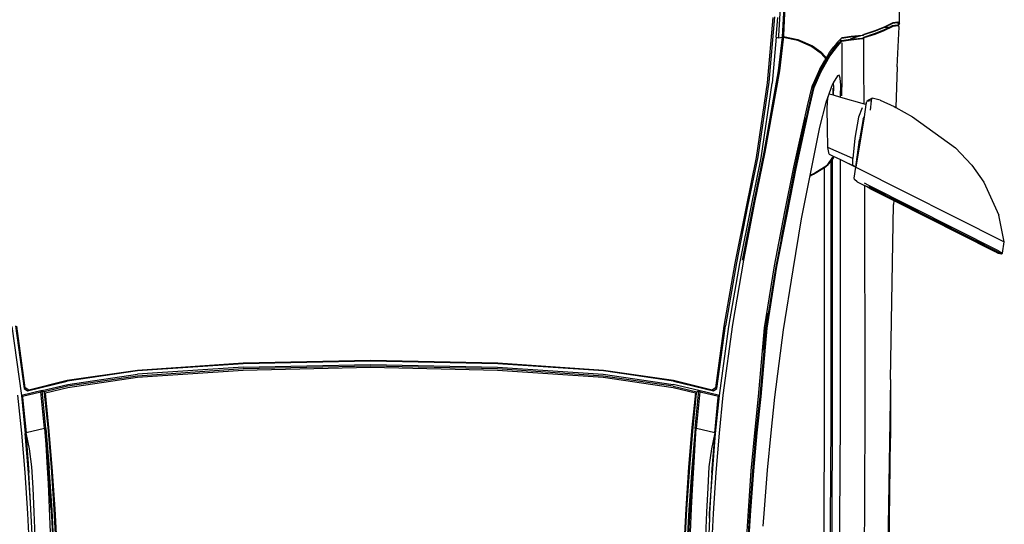
# Model space of a CAD drawing. Units: inches. Extents: x -4737294 to -4736756, y 1716389 to 1717040.
# Tile 11 of 25: x -4737176 to -4737103, y 1716559 to 1716597. Entities that reach past the tile are written whole.
import ezdxf

# ---------------------------------------------------------------- set-up
doc = ezdxf.new("R2010")
doc.units = ezdxf.units.IN
doc.header["$MEASUREMENT"] = 0
doc.layers.add('A-EQPM-VEHI', color=250, linetype='Continuous', lineweight=13)
doc.layers.add('Edges', color=250, linetype='Continuous')

# ---------------------------------------------------------------- blocks, each defined once
blk = doc.blocks.new('Nissan Qashqai pl')
at = {"layer": 'Edges'}
for p, q in [((8.8918, 12.7444), (9.0186, 12.9956)), ((9.0386, 12.9907), (8.9254, 12.7664)), ((9.0186, 12.9956), (8.9731, 12.9865)), ((9.0374, 12.9925), (9.0186, 12.9956)), ((9.0356, 12.9888), (9.0374, 12.9925)), ((9.0386, 12.9907), (9.0374, 12.9925)), ((9.0376, 12.985), (9.0386, 12.9907)), ((8.9173, 12.961), (8.9731, 12.9865)), ((9.0333, 12.9845), (8.9232, 12.7662)), ((8.9483, 12.8082), (9.0343, 12.9785)), ((9.0356, 12.9888), (9.0333, 12.9845)), ((9.0343, 12.9785), (9.0347, 12.9794)), ((9.0347, 12.9794), (9.0362, 12.9822)), ((9.0362, 12.9822), (9.037, 12.9838)), ((9.0371, 12.9841), (9.037, 12.9838)), ((9.0371, 12.9841), (9.0376, 12.985)), ((9.0376, 12.985), (9.0371, 12.9847)), ((8.8885, 12.9405), (8.9173, 12.961)), ((8.8591, 12.9127), (8.8879, 12.94)), ((8.8885, 12.9405), (8.8879, 12.94)), ((8.8066, 12.84), (8.8591, 12.9127)), ((8.7908, 12.812), (8.8066, 12.84)), ((8.6489, 12.8179), (8.5719, 12.8193)), ((8.646, 12.8153), (8.6489, 12.8179)), ((8.646, 12.8153), (8.646, 12.8153)), ((8.6472, 12.8076), (8.646, 12.8153)), ((8.647, 12.8142), (8.6498, 12.8168)), ((8.6482, 12.8067), (8.647, 12.8142)), ((8.6546, 12.7926), (8.6472, 12.8076)), ((8.655, 12.7929), (8.6482, 12.8067)), ((8.6489, 12.8179), (8.6527, 12.8156)), ((8.6498, 12.8168), (8.6524, 12.8153)), ((8.651, 12.814), (8.652, 12.815)), ((8.6524, 12.8064), (8.651, 12.814)), ((8.652, 12.815), (8.6524, 12.8153)), ((8.6534, 12.8073), (8.652, 12.815)), ((8.6524, 12.8153), (8.6527, 12.8156)), ((8.6527, 12.8156), (8.6537, 12.8167)), ((8.6608, 12.7921), (8.6534, 12.8073)), ((8.6547, 12.8176), (8.6537, 12.8167)), ((8.6537, 12.8167), (8.6537, 12.8166)), ((8.7222, 12.8144), (8.6547, 12.8176)), ((8.7222, 12.8144), (8.7908, 12.812)), ((8.7785, 12.7855), (8.7891, 12.8089)), ((8.7891, 12.8089), (8.7908, 12.812)), ((8.928, 12.7679), (8.9483, 12.8082)), ((8.9483, 12.8082), (8.9552, 12.8081)), ((9.2517, 12.8031), (8.9552, 12.8081)), ((8.655, 12.801), (8.6524, 12.8064)), ((8.6606, 12.7768), (8.6546, 12.7926)), ((8.6598, 12.7913), (8.655, 12.801)), ((8.655, 12.7929), (8.655, 12.801)), ((8.6556, 12.7918), (8.655, 12.7929)), ((8.655, 12.7922), (8.655, 12.7929)), ((8.6616, 12.7758), (8.6556, 12.7918)), ((8.6657, 12.7758), (8.6598, 12.7913)), ((8.6667, 12.7767), (8.6608, 12.7921)), ((9.2517, 12.8031), (9.351, 12.803)), ((9.2517, 12.8031), (9.5372, 12.7983)), ((9.641, 12.7991), (9.351, 12.803)), ((8.6667, 12.7584), (8.6606, 12.7768)), ((8.6675, 12.758), (8.6616, 12.7758)), ((8.6718, 12.7574), (8.6657, 12.7758)), ((8.6728, 12.7584), (8.6667, 12.7767)), ((8.7785, 12.7855), (8.7751, 12.7719)), ((8.6675, 12.758), (8.6667, 12.7584)), ((8.6679, 12.7578), (8.6675, 12.758)), ((8.6676, 12.7576), (8.6675, 12.7576)), ((8.6675, 12.7576), (8.6675, 12.7576)), ((8.6675, 12.7576), (8.6676, 12.7576)), ((8.6676, 12.7576), (8.6677, 12.7576)), ((8.6677, 12.7576), (8.6677, 12.7576)), ((8.6677, 12.7576), (8.6682, 12.7576)), ((8.6682, 12.7576), (8.6679, 12.7578)), ((8.6682, 12.7576), (8.6692, 12.7566)), ((8.6682, 12.7572), (8.6682, 12.7576)), ((8.6684, 12.7554), (8.6682, 12.7572)), ((8.6682, 12.7572), (8.6692, 12.7566)), ((8.6692, 12.7566), (8.6697, 12.7519)), ((8.6729, 12.7568), (8.6718, 12.7574)), ((8.674, 12.7578), (8.6728, 12.7584)), ((8.6733, 12.7566), (8.6729, 12.7568)), ((8.6735, 12.7544), (8.6733, 12.7566)), ((8.6742, 12.7576), (8.674, 12.7578)), ((8.6742, 12.7584), (8.6743, 12.7582)), ((8.6744, 12.755), (8.6742, 12.7576)), ((8.6744, 12.7576), (8.6742, 12.7576)), ((8.6744, 12.7578), (8.6744, 12.7576)), ((8.6773, 12.7577), (8.6744, 12.7576)), ((8.6791, 12.7578), (8.677, 12.7578)), ((8.6791, 12.7577), (8.6773, 12.7577)), ((8.7205, 12.7579), (8.6791, 12.7578)), ((8.6791, 12.7577), (8.6791, 12.7578)), ((8.6878, 12.7577), (8.6791, 12.7578)), ((8.6878, 12.7577), (8.6791, 12.7577)), ((8.6878, 12.7577), (8.6878, 12.7577)), ((8.6911, 12.7577), (8.6878, 12.7577)), ((8.7205, 12.7579), (8.6911, 12.7577)), ((8.7849, 12.7582), (8.7205, 12.7579)), ((8.7734, 12.7181), (8.7849, 12.7582)), ((8.7751, 12.7719), (8.7779, 12.7668)), ((8.7798, 12.7703), (8.7751, 12.7719)), ((8.7779, 12.7668), (8.7807, 12.763)), ((8.7798, 12.7703), (8.7807, 12.763)), ((8.7798, 12.7703), (8.7954, 12.7683)), ((8.7849, 12.7615), (8.7807, 12.763)), ((8.7849, 12.7615), (8.7858, 12.7613)), ((8.7849, 12.7582), (8.7856, 12.7608)), ((8.7858, 12.7613), (8.7856, 12.7608)), ((8.7858, 12.7613), (8.807, 12.758)), ((8.8102, 12.7568), (8.807, 12.758)), ((8.807, 12.758), (8.8918, 12.7444)), ((8.8102, 12.7568), (8.8455, 12.7506)), ((8.9171, 12.7464), (8.9233, 12.7586)), ((8.9232, 12.7662), (8.9194, 12.7588)), ((8.925, 12.762), (8.9233, 12.7586)), ((8.9233, 12.7586), (9.2886, 12.7594)), ((8.928, 12.7679), (8.925, 12.762)), ((9.2886, 12.7594), (9.4673, 12.7589)), ((9.4673, 12.7589), (9.6358, 12.7575)), ((8.6684, 12.7554), (8.6685, 12.7549)), ((8.6684, 12.755), (8.6684, 12.7554)), ((8.6703, 12.7361), (8.6684, 12.755)), ((8.6697, 12.7519), (8.6698, 12.7516)), ((8.6714, 12.7353), (8.6697, 12.7519)), ((8.6698, 12.7516), (8.6755, 12.7343)), ((8.6754, 12.7353), (8.6735, 12.7544)), ((8.6764, 12.736), (8.6744, 12.755)), ((8.7917, 12.7547), (8.8075, 12.7486)), ((8.8075, 12.7486), (8.8429, 12.7426)), ((8.8429, 12.7426), (8.8771, 12.7388)), ((8.8918, 12.7444), (8.8455, 12.7506)), ((8.8815, 12.7228), (8.892, 12.7444)), ((8.8908, 12.7421), (8.8895, 12.7393)), ((8.8906, 12.7418), (8.8895, 12.7393)), ((8.8906, 12.7418), (8.8911, 12.7428)), ((8.892, 12.7444), (8.8908, 12.7421)), ((8.8911, 12.7428), (8.8919, 12.7444)), ((8.8911, 12.7428), (8.8919, 12.7444)), ((8.8919, 12.7444), (8.8911, 12.7428)), ((8.8919, 12.7444), (8.8918, 12.7444)), ((8.892, 12.7444), (8.8919, 12.7444)), ((8.8919, 12.7444), (8.8919, 12.7444)), ((8.8919, 12.7444), (8.8919, 12.7444)), ((8.9106, 12.7413), (8.892, 12.7444)), ((8.892, 12.7444), (8.892, 12.7444)), ((8.9131, 12.7421), (8.9106, 12.7413)), ((8.9171, 12.7464), (8.9131, 12.7421)), ((8.9171, 12.7464), (8.917, 12.7468)), ((8.6727, 12.7207), (8.6703, 12.7361)), ((8.6737, 12.7197), (8.6714, 12.7353)), ((8.6755, 12.7343), (8.6754, 12.7353)), ((8.6777, 12.7196), (8.6755, 12.7343)), ((8.6764, 12.7359), (8.6764, 12.736)), ((8.6788, 12.7205), (8.6764, 12.7359)), ((8.8771, 12.7388), (8.8585, 12.6969)), ((8.8895, 12.7393), (8.8771, 12.7388)), ((8.8815, 12.7228), (8.8895, 12.7393)), ((8.6737, 12.7197), (8.6727, 12.7207)), ((8.6746, 12.7189), (8.6737, 12.7197)), ((8.6785, 12.7189), (8.6746, 12.7189)), ((8.6805, 12.7132), (8.6746, 12.7189)), ((8.6785, 12.7189), (8.6777, 12.7196)), ((8.6815, 12.7162), (8.6785, 12.7189)), ((8.687, 12.7132), (8.6788, 12.7205)), ((8.6805, 12.7132), (8.6884, 12.7071)), ((8.6815, 12.7162), (8.6818, 12.7154)), ((8.6817, 12.716), (8.6815, 12.7162)), ((8.6817, 12.716), (8.6818, 12.7154)), ((8.6859, 12.7122), (8.6817, 12.716)), ((8.6818, 12.7204), (8.7012, 12.7203)), ((8.6818, 12.7154), (8.6902, 12.7081)), ((8.6927, 12.7071), (8.6859, 12.7122)), ((8.7042, 12.7002), (8.687, 12.7132)), ((8.6917, 12.7071), (8.6884, 12.7071)), ((8.698, 12.6996), (8.6884, 12.7071)), ((8.6902, 12.7081), (8.6917, 12.7071)), ((8.6917, 12.7071), (8.7075, 12.6955)), ((8.6927, 12.7071), (8.6923, 12.7071)), ((8.7032, 12.6992), (8.6927, 12.7071)), ((8.7012, 12.7203), (8.7012, 12.7203)), ((8.7012, 12.7203), (8.7026, 12.7203)), ((8.7026, 12.7203), (8.7026, 12.7203)), ((8.7026, 12.7203), (8.7072, 12.7203)), ((8.7072, 12.7203), (8.7072, 12.7203)), ((8.7072, 12.7203), (8.7273, 12.7202)), ((8.7273, 12.7202), (8.7273, 12.7201)), ((8.7273, 12.7202), (8.7354, 12.7202)), ((8.7354, 12.7201), (8.7354, 12.7202)), ((8.7354, 12.7202), (8.742, 12.7202)), ((8.7415, 12.7177), (8.7361, 12.7158)), ((8.7361, 12.7158), (8.7373, 12.7128)), ((8.7373, 12.7128), (8.7492, 12.7059)), ((8.7534, 12.7185), (8.7415, 12.7177)), ((8.742, 12.7201), (8.742, 12.7202)), ((8.742, 12.7202), (8.742, 12.7201)), ((8.742, 12.7202), (8.742, 12.7202)), ((8.742, 12.7202), (8.7426, 12.7202)), ((8.7426, 12.7201), (8.7426, 12.7202)), ((8.7426, 12.7202), (8.7433, 12.7202)), ((8.7433, 12.7201), (8.7433, 12.7202)), ((8.7433, 12.7202), (8.7711, 12.7201)), ((8.7711, 12.7201), (8.7516, 12.72)), ((8.7718, 12.7181), (8.7534, 12.7185)), ((8.7698, 12.7058), (8.7734, 12.7181)), ((8.7734, 12.7181), (8.7718, 12.7181)), ((8.8734, 12.7057), (8.8793, 12.7181)), ((8.8793, 12.7181), (8.8815, 12.7228)), ((9.3194, 12.7179), (8.8793, 12.7181)), ((9.4919, 12.7173), (9.3194, 12.7179)), ((9.6538, 12.7157), (9.4919, 12.7173)), ((8.697, 12.685), (8.7055, 12.6927)), ((8.6979, 12.6839), (8.7062, 12.6915)), ((8.7071, 12.6942), (8.698, 12.6996)), ((8.7062, 12.6915), (8.6987, 12.6845)), ((8.7302, 12.684), (8.7032, 12.6992)), ((8.7312, 12.6851), (8.7042, 12.7002)), ((8.7055, 12.6927), (8.7071, 12.6942)), ((8.7062, 12.6915), (8.7067, 12.6919)), ((8.7067, 12.6919), (8.7083, 12.6934)), ((8.7071, 12.6942), (8.7083, 12.6934)), ((8.7075, 12.6955), (8.7346, 12.6806)), ((8.7083, 12.6934), (8.7083, 12.6934)), ((8.7083, 12.6934), (8.7083, 12.6934)), ((8.7102, 12.6923), (8.7083, 12.6934)), ((8.7083, 12.6934), (8.7083, 12.6934)), ((8.7108, 12.6919), (8.7102, 12.6923)), ((8.7102, 12.6923), (8.7102, 12.6923)), ((8.7257, 12.6833), (8.7108, 12.6919)), ((8.7248, 12.6836), (8.7108, 12.6919)), ((8.7492, 12.7059), (8.7572, 12.7062)), ((8.7492, 12.7059), (8.7524, 12.704)), ((8.7524, 12.704), (8.7828, 12.6934)), ((8.7572, 12.7062), (8.7698, 12.7058)), ((8.7698, 12.7057), (8.7583, 12.706)), ((8.7678, 12.6988), (8.7698, 12.7057)), ((8.7748, 12.6967), (8.7678, 12.6988)), ((8.7698, 12.7057), (8.7698, 12.7058)), ((8.7916, 12.6954), (8.7748, 12.6967)), ((8.7828, 12.6934), (8.8245, 12.6828)), ((8.8259, 12.6959), (8.7916, 12.6954)), ((8.8585, 12.6969), (8.8259, 12.6959)), ((8.87, 12.6987), (8.8585, 12.6969)), ((8.87, 12.6987), (8.8734, 12.7057)), ((8.8734, 12.7057), (8.8768, 12.7057)), ((8.8751, 12.7054), (8.8768, 12.7057)), ((8.8893, 12.6956), (8.8751, 12.7054)), ((8.8768, 12.7057), (8.879, 12.704)), ((8.879, 12.704), (9.3198, 12.7039)), ((8.879, 12.704), (8.881, 12.7023)), ((9.3225, 12.7021), (8.881, 12.7023)), ((8.881, 12.7023), (8.8893, 12.6956)), ((8.8893, 12.6956), (8.9021, 12.6745)), ((8.8913, 12.6936), (8.8893, 12.6956)), ((8.8927, 12.6913), (8.8913, 12.6936)), ((9.3224, 12.6911), (8.8927, 12.6913)), ((8.9041, 12.6725), (8.8927, 12.6913)), ((9.3198, 12.7039), (9.4922, 12.7033)), ((9.3225, 12.6911), (9.3224, 12.6911)), ((9.4936, 12.7013), (9.3225, 12.7021)), ((9.4936, 12.6904), (9.3225, 12.6911)), ((9.4922, 12.7033), (9.654, 12.7018)), ((9.6552, 12.6997), (9.4936, 12.7013)), ((9.6552, 12.6888), (9.4936, 12.6904)), ((8.6864, 12.6706), (8.697, 12.685)), ((8.6875, 12.6698), (8.6979, 12.6839)), ((8.6924, 12.676), (8.6883, 12.6704)), ((8.6987, 12.6845), (8.6924, 12.676)), ((8.6924, 12.676), (8.6924, 12.6762)), ((8.7257, 12.6833), (8.7248, 12.6836)), ((8.7257, 12.6832), (8.7257, 12.6833)), ((8.7257, 12.6832), (8.7508, 12.672)), ((8.7529, 12.6741), (8.7302, 12.684)), ((8.7574, 12.6737), (8.7312, 12.6851)), ((8.7346, 12.6806), (8.7491, 12.6738)), ((8.7346, 12.6806), (8.7577, 12.6709)), ((8.7508, 12.672), (8.7491, 12.6738)), ((8.7491, 12.6738), (8.7576, 12.6699)), ((8.7529, 12.6741), (8.7577, 12.6709)), ((8.757, 12.6724), (8.7529, 12.6741)), ((8.7931, 12.6653), (8.7574, 12.6737)), ((8.8245, 12.6828), (8.9063, 12.6663)), ((8.9021, 12.6745), (8.9063, 12.6663)), ((8.6759, 12.6459), (8.6864, 12.6706)), ((8.6772, 12.6454), (8.6875, 12.6698)), ((8.6883, 12.6704), (8.6777, 12.6457)), ((8.7532, 12.6708), (8.7508, 12.672)), ((8.7575, 12.6698), (8.7532, 12.6708)), ((8.7587, 12.672), (8.757, 12.6724)), ((8.7576, 12.6699), (8.7575, 12.6698)), ((8.7881, 12.6621), (8.7575, 12.6698)), ((8.7582, 12.6707), (8.7576, 12.6699)), ((8.7577, 12.6709), (8.7582, 12.6707)), ((8.759, 12.6717), (8.7582, 12.6707)), ((8.7587, 12.672), (8.759, 12.6717)), ((8.7591, 12.6719), (8.7587, 12.672)), ((8.7591, 12.6719), (8.759, 12.6717)), ((8.7925, 12.664), (8.7591, 12.6719)), ((8.8918, 12.6392), (8.7881, 12.6621)), ((8.8941, 12.6418), (8.7925, 12.664)), ((8.8942, 12.6432), (8.7931, 12.6653)), ((8.8083, 12.6591), (8.8954, 12.6403)), ((8.9075, 12.6661), (8.9041, 12.6725)), ((8.9063, 12.6663), (8.9075, 12.6661)), ((8.9075, 12.6661), (8.9087, 12.6658)), ((8.9087, 12.6658), (8.9797, 12.6518)), ((8.6716, 12.6242), (8.6759, 12.6459)), ((8.6772, 12.6454), (8.6721, 12.6201)), ((8.6777, 12.6457), (8.6727, 12.6213)), ((9.0601, 12.6092), (8.8941, 12.6418)), ((8.9696, 12.6285), (8.8942, 12.6432)), ((8.8961, 12.6401), (8.9704, 12.6257)), ((8.9797, 12.6518), (9.0656, 12.6372)), ((8.6197, 12.6241), (8.6683, 12.6215)), ((8.671, 12.6214), (8.6716, 12.6242)), ((8.9679, 12.6241), (8.8918, 12.6392)), ((9.0591, 12.6065), (8.9679, 12.6241)), ((9.06, 12.6106), (8.9696, 12.6285)), ((8.9704, 12.6257), (8.9708, 12.6256)), ((8.9708, 12.6256), (9.0143, 12.6169)), ((9.0656, 12.6372), (9.1676, 12.6212)), ((8.6721, 12.6201), (8.6204, 12.6229)), ((8.622, 12.6161), (8.6699, 12.6132)), ((8.6375, 12.6066), (8.7481, 12.5968)), ((8.6721, 12.6093), (8.6387, 12.6123)), ((8.6683, 12.6215), (8.671, 12.6214)), ((8.6699, 12.6132), (8.6721, 12.613)), ((8.671, 12.6214), (8.6721, 12.6201)), ((8.6727, 12.6213), (8.6721, 12.6201)), ((8.6733, 12.6129), (8.6721, 12.6201)), ((8.7287, 12.6134), (8.6721, 12.6201)), ((8.6721, 12.6127), (8.6721, 12.613)), ((8.6721, 12.613), (8.6733, 12.6129)), ((8.6721, 12.6093), (8.6733, 12.6129)), ((8.6721, 12.6093), (8.7496, 12.6025)), ((8.6727, 12.6213), (8.6753, 12.621)), ((8.6753, 12.621), (8.7292, 12.6146)), ((8.8666, 12.5888), (8.7287, 12.6134)), ((8.7292, 12.6146), (8.8666, 12.5901)), ((9.1644, 12.5938), (9.06, 12.6106)), ((9.1645, 12.5924), (9.0601, 12.6092)), ((9.1676, 12.6212), (9.2814, 12.6065)), ((8.6386, 12.6037), (8.7491, 12.594)), ((8.7481, 12.5968), (8.8745, 12.5782)), ((8.7491, 12.594), (8.8754, 12.5755)), ((8.8761, 12.5839), (8.7496, 12.6025)), ((8.8666, 12.5901), (8.9521, 12.5726)), ((9.1639, 12.5895), (9.0591, 12.6065)), ((9.1393, 12.5951), (9.1647, 12.591)), ((9.2803, 12.5836), (9.1644, 12.5938)), ((9.2804, 12.5821), (9.1645, 12.5924)), ((9.1647, 12.591), (9.1668, 12.5908)), ((9.1668, 12.5908), (9.2019, 12.5877)), ((9.2814, 12.6065), (9.3416, 12.5999)), ((9.3416, 12.5999), (9.4048, 12.5941)), ((9.4048, 12.5941), (9.471, 12.5888)), ((8.9522, 12.5713), (8.8666, 12.5888)), ((8.8745, 12.5782), (8.9583, 12.5609)), ((8.8754, 12.5755), (8.9591, 12.5583)), ((8.9598, 12.5666), (8.8761, 12.5839)), ((9.2801, 12.5794), (9.1639, 12.5895)), ((9.3418, 12.5729), (9.2801, 12.5794)), ((9.3418, 12.5771), (9.2803, 12.5836)), ((9.3419, 12.5756), (9.2804, 12.5821)), ((9.4062, 12.5713), (9.3418, 12.5771)), ((9.4063, 12.5699), (9.3419, 12.5756)), ((9.471, 12.5888), (9.4997, 12.5869)), ((8.9521, 12.5726), (9.0495, 12.5536)), ((9.0497, 12.5523), (8.9522, 12.5713)), ((8.9583, 12.5609), (9.0538, 12.5419)), ((8.9591, 12.5583), (9.0546, 12.5394)), ((9.0552, 12.5477), (8.9598, 12.5666)), ((9.4064, 12.5671), (9.3418, 12.5729)), ((9.4735, 12.5663), (9.4062, 12.5713)), ((9.4736, 12.5648), (9.4063, 12.5699)), ((9.4739, 12.5621), (9.4064, 12.5671)), ((9.5437, 12.5619), (9.4735, 12.5663)), ((9.5438, 12.5605), (9.4736, 12.5648)), ((9.5443, 12.5579), (9.4739, 12.5621)), ((9.0495, 12.5536), (9.1584, 12.5351)), ((9.0538, 12.5419), (9.1605, 12.5233)), ((9.1617, 12.5292), (9.0552, 12.5477)), ((9.0546, 12.5394), (9.1612, 12.5208)), ((9.1584, 12.5351), (9.2783, 12.5191)), ((9.2669, 12.5088), (9.1605, 12.5233)), ((9.2789, 12.5131), (9.1617, 12.5292)), ((9.1612, 12.5208), (9.2656, 12.5065)), ((9.2656, 12.5065), (9.2669, 12.5088)), ((9.2656, 12.5065), (9.2694, 12.5006)), ((9.2707, 12.5028), (9.2669, 12.5088)), ((9.2789, 12.5131), (9.2704, 12.4783)), ((9.2724, 12.4804), (9.2799, 12.5114)), ((9.2783, 12.5191), (9.3422, 12.5126)), ((9.2799, 12.5114), (9.2789, 12.5131)), ((9.3427, 12.5066), (9.2789, 12.5131)), ((9.2819, 12.5112), (9.2799, 12.5114)), ((9.2803, 12.5116), (9.2822, 12.5118)), ((9.3418, 12.5051), (9.2819, 12.5112)), ((9.3422, 12.5126), (9.4088, 12.507)), ((9.4093, 12.5011), (9.3427, 12.5066)), ((9.4088, 12.507), (9.4782, 12.5024)), ((9.2694, 12.5006), (9.2535, 12.4354)), ((9.2543, 12.4356), (9.2707, 12.5028)), ((9.2707, 12.5028), (9.2694, 12.5006)), ((9.3418, 12.5051), (9.3346, 12.4741)), ((9.342, 12.5059), (9.3418, 12.5051)), ((9.3687, 12.5), (9.342, 12.5059)), ((9.4087, 12.5003), (9.342, 12.5059)), ((9.3992, 12.496), (9.3687, 12.5)), ((9.4347, 12.494), (9.3992, 12.496)), ((9.4087, 12.5003), (9.4688, 12.4968)), ((9.4785, 12.4965), (9.4093, 12.5011)), ((9.4761, 12.4919), (9.4347, 12.494)), ((9.4688, 12.4968), (9.4789, 12.4964)), ((9.5168, 12.4903), (9.4761, 12.4919)), ((9.4782, 12.5024), (9.5503, 12.4987)), ((9.4789, 12.4964), (9.4785, 12.4965)), ((9.4862, 12.4961), (9.4785, 12.4965)), ((9.4789, 12.4964), (9.4862, 12.4961)), ((9.4862, 12.4961), (9.514, 12.4949)), ((9.2704, 12.4783), (9.2598, 12.4348)), ((9.2629, 12.435), (9.2726, 12.4746)), ((9.2724, 12.4804), (9.2704, 12.4783)), ((9.2726, 12.4746), (9.2704, 12.4783)), ((9.3346, 12.4718), (9.2704, 12.4783)), ((9.3346, 12.4741), (9.2724, 12.4804)), ((9.2746, 12.4744), (9.2726, 12.4746)), ((9.333, 12.4685), (9.2746, 12.4744)), ((9.3346, 12.4741), (9.3344, 12.4733)), ((9.3344, 12.4733), (9.4017, 12.4677)), ((9.3344, 12.4733), (9.3611, 12.4715)), ((9.2649, 12.4348), (9.2741, 12.4725)), ((9.2741, 12.4725), (9.3326, 12.4666)), ((9.3326, 12.4666), (9.4, 12.4609)), ((9.4004, 12.4629), (9.333, 12.4685)), ((9.3346, 12.4718), (9.4018, 12.4661)), ((9.3611, 12.4715), (9.3918, 12.4695)), ((9.3918, 12.4695), (9.4276, 12.4674)), ((9.4, 12.4609), (9.4706, 12.4561)), ((9.4709, 12.4581), (9.4004, 12.4629)), ((9.4017, 12.4677), (9.472, 12.463)), ((9.4018, 12.4661), (9.472, 12.4614)), ((9.4276, 12.4674), (9.4694, 12.4654)), ((9.4694, 12.4654), (9.5105, 12.4637)), ((9.5446, 12.4542), (9.4709, 12.4581)), ((9.472, 12.463), (9.5454, 12.4591)), ((9.472, 12.4614), (9.5454, 12.4576)), ((9.4706, 12.4561), (9.5443, 12.4522)), ((9.2535, 12.4354), (9.2362, 12.3167)), ((9.2543, 12.4356), (9.2371, 12.3169)), ((9.2426, 12.3164), (9.2598, 12.4348)), ((9.2629, 12.435), (9.2457, 12.3164)), ((9.2476, 12.3163), (9.2649, 12.4348)), ((9.2362, 12.3167), (9.2241, 12.1376)), ((9.2371, 12.3169), (9.2249, 12.1376)), ((9.2305, 12.1375), (9.2426, 12.3164)), ((9.2457, 12.3164), (9.2335, 12.1374)), ((9.2355, 12.1374), (9.2476, 12.3163)), ((9.2241, 12.1376), (9.2195, 11.9221)), ((9.2249, 12.1376), (9.2203, 11.9221)), ((9.2259, 11.9221), (9.2305, 12.1375)), ((9.2335, 12.1374), (9.2289, 11.9221)), ((9.2308, 11.9221), (9.2355, 12.1374)), ((9.2195, 11.9221), (9.2241, 11.7066)), ((9.2203, 11.9221), (9.2249, 11.7065)), ((9.2305, 11.7067), (9.2259, 11.9221)), ((9.2289, 11.9221), (9.2335, 11.7067)), ((9.2355, 11.7068), (9.2308, 11.9221)), ((9.2241, 11.7066), (9.2362, 11.5274)), ((9.2249, 11.7065), (9.2371, 11.5273)), ((9.2305, 11.7067), (9.2426, 11.5277)), ((9.2335, 11.7067), (9.2457, 11.5277)), ((9.2476, 11.5278), (9.2355, 11.7068)), ((9.2362, 11.5274), (9.2535, 11.4087)), ((9.2371, 11.5273), (9.2543, 11.4085)), ((9.2598, 11.4093), (9.2426, 11.5277)), ((9.2457, 11.5277), (9.2629, 11.4092)), ((9.2649, 11.4094), (9.2476, 11.5278)), ((9.2535, 11.4087), (9.2694, 11.3436)), ((9.2707, 11.3414), (9.2543, 11.4085)), ((9.2704, 11.3659), (9.2598, 11.4093)), ((9.2629, 11.4092), (9.2726, 11.3695)), ((9.2741, 11.3716), (9.2649, 11.4094)), ((9.5443, 11.3919), (9.4706, 11.388)), ((9.4709, 11.3861), (9.5446, 11.39)), ((9.3326, 11.3776), (9.2741, 11.3716)), ((9.2746, 11.3697), (9.333, 11.3757)), ((9.4, 11.3832), (9.3326, 11.3776)), ((9.333, 11.3757), (9.4004, 11.3813)), ((9.4017, 11.3765), (9.3344, 11.3708)), ((9.3611, 11.3727), (9.3344, 11.3708)), ((9.3346, 11.3724), (9.4018, 11.378)), ((9.3918, 11.3747), (9.3611, 11.3727)), ((9.4276, 11.3767), (9.3918, 11.3747)), ((9.4706, 11.388), (9.4, 11.3832)), ((9.4004, 11.3813), (9.4709, 11.3861)), ((9.472, 11.3812), (9.4017, 11.3765)), ((9.472, 11.3828), (9.4018, 11.378)), ((9.4694, 11.3788), (9.4276, 11.3767)), ((9.5105, 11.3805), (9.4694, 11.3788)), ((9.5454, 11.3866), (9.472, 11.3828)), ((9.472, 11.3812), (9.5454, 11.3851)), ((9.3346, 11.3724), (9.2704, 11.3659)), ((9.2704, 11.3659), (9.2726, 11.3695)), ((9.2704, 11.3659), (9.2724, 11.3637)), ((9.2704, 11.3659), (9.2789, 11.331)), ((9.3346, 11.37), (9.2724, 11.3637)), ((9.2799, 11.3328), (9.2724, 11.3637)), ((9.2726, 11.3695), (9.2746, 11.3697)), ((9.3344, 11.3708), (9.3346, 11.37)), ((9.3346, 11.37), (9.3418, 11.3391)), ((9.2694, 11.3436), (9.2656, 11.3376)), ((9.2669, 11.3354), (9.2707, 11.3414)), ((9.2694, 11.3436), (9.2707, 11.3414)), ((9.342, 11.3383), (9.3687, 11.3441)), ((9.342, 11.3383), (9.4087, 11.3438)), ((9.4093, 11.3431), (9.3427, 11.3375)), ((9.3687, 11.3441), (9.3992, 11.3482)), ((9.3992, 11.3482), (9.4347, 11.3502)), ((9.4605, 11.3465), (9.4087, 11.3438)), ((9.4782, 11.3418), (9.4088, 11.3371)), ((9.4605, 11.3465), (9.4093, 11.3431)), ((9.4347, 11.3502), (9.4761, 11.3522)), ((9.514, 11.3492), (9.4605, 11.3465)), ((9.4761, 11.3522), (9.5168, 11.3539)), ((9.5503, 11.3455), (9.4782, 11.3418)), ((9.1605, 11.3208), (9.2669, 11.3354)), ((9.2656, 11.3376), (9.1612, 11.3233)), ((9.1617, 11.315), (9.2789, 11.331)), ((9.2669, 11.3354), (9.2656, 11.3376)), ((9.3422, 11.3316), (9.2783, 11.3251)), ((9.2789, 11.331), (9.3427, 11.3375)), ((9.2789, 11.331), (9.2799, 11.3327)), ((9.2799, 11.3328), (9.2819, 11.333)), ((9.2799, 11.3327), (9.2799, 11.3328)), ((9.2799, 11.3327), (9.2811, 11.3325)), ((9.2819, 11.333), (9.3418, 11.3391)), ((9.3418, 11.3391), (9.342, 11.3383)), ((9.4088, 11.3371), (9.3422, 11.3316))]:
    blk.add_line(p, q, dxfattribs=at)
blk = doc.blocks.new('car')
blk.add_blockref('Nissan Qashqai pl', (-9.7433, -11.9151))

msp = doc.modelspace()

# ---------------------------------------------------------------- block references
at = {"layer": 'A-EQPM-VEHI', "xscale": 43.56002006885659, "yscale": 43.56002006885659, "zscale": 43.56002006885659, "rotation": 270}
msp.add_blockref('car', (-4737150.017, 1716548.61), dxfattribs=at)

doc.saveas('drawing.dxf')
